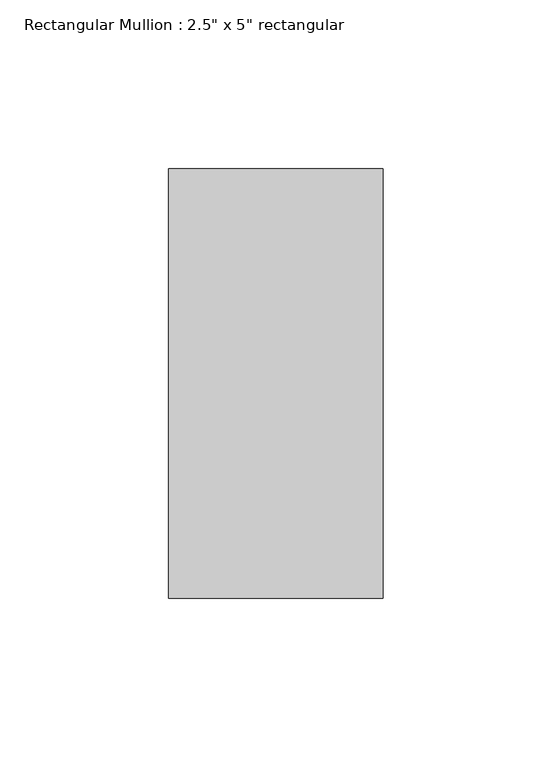
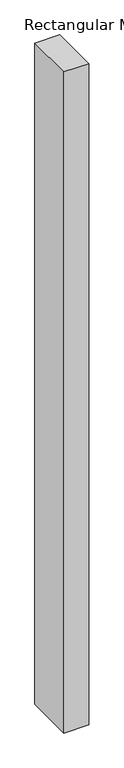
"""IFC4 building model written with IfcOpenShell, lengths in millimetres: member geometry."""

from ifc_helpers import new_model, si_unit, frame, origin, place, context, project, spatial, polyline, outline, extrude, source, transform, mapped, element, save


def member_eeabd68d(model_context):
    return source(origin(), model_context, "Body", "SweptSolid", [
        extrude(outline(polyline([(31.75, 63.5), (31.75, -63.5), (-31.75, -63.5), (-31.75, 63.5), (31.75, 63.5)])), frame((0.0, 0.0, -1771.500021), z_axis=(0.0, 0.0, 1.0), x_axis=(1.0, 0.0, 0.0)), (0.0, 0.0, 1.0), 1771.500021),
    ])


if __name__ == "__main__":
    model = new_model("IFC4")
    model_context = context("Model", 3, world=origin())
    ifc_project = project(units=[si_unit("LENGTHUNIT", "METRE", prefix="MILLI")], contexts=[model_context])
    site = spatial("IfcSite", under=ifc_project)
    building = spatial("IfcBuilding", under=site)
    placement = place(None, origin())
    member_shape = member_eeabd68d(model_context)
    element("IfcMember", 1, ObjectType="Rectangular Mullion : 2.5\" x 5\" rectangular", at=placement, inside=building, context=model_context, shape_type="MappedRepresentation", body=[
        mapped(member_shape, transform((0.0, 0.0, 0.0), x_axis=(1.0, 0.0, 0.0), y_axis=(0.0, 1.0, 0.0), z_axis=(0.0, 0.0, 1.0))),
    ])
    save(model, "model.ifc")

# Revit data of these elements
# Type "Rectangular Mullion : 2.5\" x 5\" rectangular"
#   built-in parameter 1007304 = 0.416667 (stored number, unit not read)
#   built-in parameter 1007301 = 0.104167 (stored number, unit not read)
#   built-in parameter 1007300 = 0.104167 (stored number, unit not read)
# Element 1 (IfcMember, "Rectangular Mullion : 2.5\" x 5\" rectangular")
#   Materials on its faces: "Aluminum"
# Materials
#   "Aluminum": class "Metal", colour RGB 247 247 247, transparency 0, Description = "Aluminum 6061", Cost = 0
